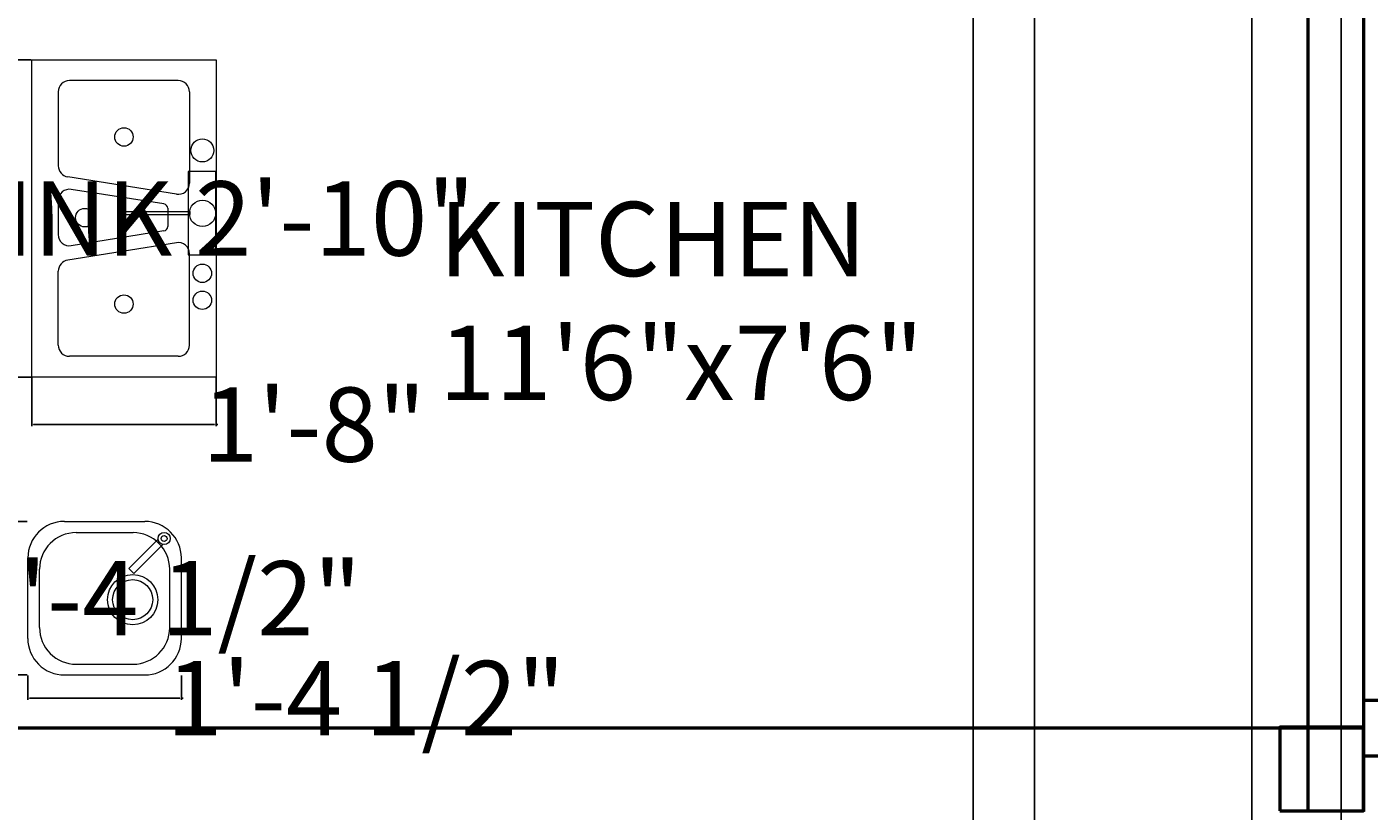
# Model space of a CAD drawing. Units: inches. Extents: x 1305 to 1889, y -508 to -5.
# Tile 3 of 8: x 1403 to 1548, y -389 to -305. Entities that reach past the tile are written whole.
import ezdxf

# ---------------------------------------------------------------- set-up
doc = ezdxf.new("R2010")
doc.units = ezdxf.units.IN
doc.header["$MEASUREMENT"] = 0
for name, color, linetype, lineweight in [('A-ANNO-DIMS', 2, 'Continuous', 18), ('A-AREA-IDEN', 7, 'Continuous', 25), ('A-COLS', 7, 'Continuous', 50), ('A-FLOR-FIXT', 9, 'Continuous', 18), ('A-WALL', 7, 'Continuous', 50)]:
    doc.layers.add(name, color=color, linetype=linetype, lineweight=lineweight)
doc.styles.get("Standard").update_dxf_attribs({"font": 'arial.ttf', "height": 8})
doc.dimstyles.get("Standard").update_dxf_attribs({"dimtxt": 0.18, "dimasz": 0.18, "dimexe": 0.18, "dimexo": 0.0625, "dimgap": 0.09, "dimtad": 0, "dimtih": 1, "dimtoh": 1, "dimzin": 0, "dimdsep": 46, "dimlunit": 4, "dimtxsty": 'Standard', "dimcen": 0.09, "dimadec": 0, "dimazin": 0, "dimtfac": 1, "dimtofl": 0, "dimtmove": 0, "dimatfit": 3, "dimfxl": 1, "dimtolj": 1, "dimtzin": 0, "dimarcsym": 0})

# ---------------------------------------------------------------- blocks, each defined once
blk = doc.blocks.new('A$C27EB6A15')
for p, q in [((0, 0), (0, 644.7)), ((0, 644.7), (1110.1, 644.7)), ((682.1, 643.4), (390.6, 643.4)), ((390.6, 643.4), (390.6, 547.6)), ((682.1, 547.6), (682.1, 643.4)), ((1110.1, 644.7), (1110.1, 0)), ((111.7, 551.5), (431.6, 551.5)), ((390.6, 547.6), (682.1, 547.6)), ((530.7, 328), (530.7, 553.3)), ((541.9, 552.9), (541.9, 328)), ((998.4, 551.5), (678.5, 551.5)), ((72.5, 512.3), (72.5, 132)), ((470.2, 506.2), (409.5, 125.9)), ((519.5, 475.4), (583.2, 475.4)), ((639.9, 506.2), (700.6, 125.9)), ((1037.5, 512.3), (1037.5, 132)), ((504.1, 462.2), (453.4, 137.6)), ((598.6, 462.2), (650.4, 137.8)), ((541.9, 328), (530.7, 328)), ((111.7, 92.9), (370.9, 92.9)), ((492.1, 92.5), (611.7, 92.5)), ((998.4, 92.9), (739.2, 92.9)), ((1110.1, 0), (0, 0))]:
    blk.add_line(p, q)
for centre, radius in [((317, 596.6), 40.3), ((537.2, 597.3), 45.9), ((747.1, 596.6), 32.3), ((841.3, 596.6), 32.3), ((269.9, 322.4), 32.3), ((854.7, 322.4), 32.3), ((552.2, 185.3), 32.3)]:
    blk.add_circle(centre, radius)
for centre, radius, start, end in [((111.7, 512.3), 39.1, 90, 180), ((431.6, 512.3), 39.1, 350.9343, 90), ((538.2, 591.7), 39.2, 259.3674, 275.2446), ((678.5, 512.3), 39.1, 90, 189.0657), ((998.4, 512.3), 39.1, 0, 90), ((519.5, 459.7), 15.7, 90, 171.1312), ((583.2, 459.7), 15.7, 9.0657, 90), ((111.7, 132), 39.1, 180, 270), ((370.9, 132), 39.1, 270, 350.9343), ((492.1, 131.6), 39.1, 171.1312, 270), ((611.7, 131.6), 39.1, 270, 9.0657), ((739.2, 132), 39.1, 189.0657, 270), ((998.4, 132), 39.1, 270, 0)]:
    blk.add_arc(centre, radius, start, end)
blk = doc.blocks.new('A$C027E3DAA')
for p, q in [((320, 419.7), (100, 419.7)), ((142.2, 289.7), (62.9, 369.3)), ((290.5, 387.8), (130.7, 387.8)), ((48.5, 356.2), (128.4, 276)), ((0, 100), (0, 319.7)), ((420, 100), (420, 319.7)), ((30.7, 132), (30.7, 287.8)), ((128.4, 276), (142.2, 289.7)), ((390.5, 132), (390.5, 287.8)), ((290.5, 32), (130.7, 32)), ((320, 0), (100, 0))]:
    blk.add_line(p, q)
for centre, radius in [((46.7, 372.6), 16.5), ((46.7, 372.6), 8.24), ((214, 286.7), 68.5), ((214, 286.7), 54.8)]:
    blk.add_circle(centre, radius)
for centre, start, end in [((100, 319.7), 90, 180), ((320, 319.7), 0, 90), ((130.7, 287.8), 90, 180), ((290.5, 287.8), 0, 90), ((130.7, 132), 180, 270), ((290.5, 132), 270, 0), ((100, 100), 180, 270), ((320, 100), 270, 0)]:
    blk.add_arc(centre, 100, start, end)
blk = doc.blocks.new('COL-9X9')
blk.add_lwpolyline([(0, 0), (9, 0), (9, 9), (0, 9)], close=True)
blk = doc.blocks.new('*D34')
at = {"layer": 'A-ANNO-DIMS', "color": 0, "lineweight": -2, "transparency": 16777216}
for p, q in [((1403.25, -358), (1400.66, -358)), ((1400.84, -358.18), (1400.84, -362.04)), ((1400.84, -374.35), (1400.84, -370.49)), ((1403.25, -374.53), (1400.66, -374.53))]:
    blk.add_line(p, q, dxfattribs=at)
at = {"layer": 'A-ANNO-DIMS', "color": 0, "transparency": 16777216}
for points in [[(1400.81, -358.18), (1400.87, -358.18), (1400.84, -358)], [(1400.81, -374.35), (1400.87, -374.35), (1400.84, -374.53)]]:
    blk.add_solid(points, dxfattribs=at)
at = {"layer": 'Defpoints', "color": 0, "transparency": 16777216}
for p in [(1403.32, -358), (1400.84, -374.53), (1403.32, -374.53)]:
    blk.add_point(p, dxfattribs=at)
at = {"layer": 'A-ANNO-DIMS', "color": 0, "transparency": 16777216, "insert": (1400.84, -366.27), "char_height": 8, "attachment_point": 5}
blk.add_mtext('\\A1;BASIN 1\'-4 1/2"', dxfattribs=at)
blk = doc.blocks.new('*D35')
at = {"layer": 'A-ANNO-DIMS', "color": 0, "lineweight": -2, "transparency": 16777216}
for p, q in [((1403.32, -374.6), (1403.32, -377.2)), ((1419.84, -374.6), (1419.84, -377.2)), ((1403.5, -377.02), (1419.66, -377.02)), ((1419.84, -377.02), (1420.02, -377.02))]:
    blk.add_line(p, q, dxfattribs=at)
at = {"layer": 'A-ANNO-DIMS', "color": 0, "transparency": 16777216}
for points in [[(1403.5, -376.99), (1403.5, -377.05), (1403.32, -377.02)], [(1419.66, -376.99), (1419.66, -377.05), (1419.84, -377.02)]]:
    blk.add_solid(points, dxfattribs=at)
at = {"layer": 'Defpoints', "color": 0, "transparency": 16777216}
for p in [(1403.32, -374.53), (1419.84, -374.53), (1419.84, -377.02)]:
    blk.add_point(p, dxfattribs=at)
at = {"layer": 'A-ANNO-DIMS', "color": 0, "transparency": 16777216, "insert": (1439.69, -377.02), "char_height": 8, "attachment_point": 5}
blk.add_mtext('\\A1;1\'-4 1/2"', dxfattribs=at)
blk = doc.blocks.new('*D44')
at = {"layer": 'A-ANNO-DIMS', "color": 0, "lineweight": -2, "transparency": 16777216}
for p, q in [((1403.68, -308.29), (1398.44, -308.29)), ((1398.62, -308.47), (1398.62, -321.14)), ((1398.62, -342.27), (1398.62, -329.59)), ((1403.68, -342.45), (1398.44, -342.45))]:
    blk.add_line(p, q, dxfattribs=at)
at = {"layer": 'A-ANNO-DIMS', "color": 0, "transparency": 16777216}
for points in [[(1398.59, -308.47), (1398.65, -308.47), (1398.62, -308.29)], [(1398.59, -342.27), (1398.65, -342.27), (1398.62, -342.45)]]:
    blk.add_solid(points, dxfattribs=at)
at = {"layer": 'Defpoints', "color": 0, "transparency": 16777216}
for p in [(1403.74, -308.29), (1398.62, -342.45), (1403.74, -342.45)]:
    blk.add_point(p, dxfattribs=at)
at = {"layer": 'A-ANNO-DIMS', "color": 0, "transparency": 16777216, "insert": (1398.62, -325.37), "char_height": 8, "attachment_point": 5}
blk.add_mtext('\\A1;KITCHEN SINK 2\'-10"', dxfattribs=at)
blk = doc.blocks.new('*D45')
at = {"layer": 'A-ANNO-DIMS', "color": 0, "lineweight": -2, "transparency": 16777216}
for p, q in [((1403.74, -342.51), (1403.74, -347.75)), ((1423.58, -342.51), (1423.58, -347.75)), ((1403.92, -347.57), (1423.4, -347.57)), ((1423.58, -347.57), (1423.76, -347.57))]:
    blk.add_line(p, q, dxfattribs=at)
at = {"layer": 'A-ANNO-DIMS', "color": 0, "transparency": 16777216}
for points in [[(1403.92, -347.54), (1403.92, -347.6), (1403.74, -347.57)], [(1423.4, -347.54), (1423.4, -347.6), (1423.58, -347.57)]]:
    blk.add_solid(points, dxfattribs=at)
at = {"layer": 'Defpoints', "color": 0, "transparency": 16777216}
for p in [(1403.74, -342.45), (1423.58, -342.45), (1423.58, -347.57)]:
    blk.add_point(p, dxfattribs=at)
at = {"layer": 'A-ANNO-DIMS', "color": 0, "transparency": 16777216, "insert": (1434.11, -347.57), "char_height": 8, "attachment_point": 5}
blk.add_mtext('\\A1;1\'-8"', dxfattribs=at)
blk = doc.blocks.new('*D55')
at = {"layer": 'A-ANNO-DIMS', "color": 0, "lineweight": -2, "transparency": 16777216}
for p, q in [((1511.68, -135.63), (1511.68, -493.26)), ((1544.68, -146.13), (1544.68, -493.26)), ((1511.86, -493.08), (1517.39, -493.08)), ((1544.5, -493.08), (1538.97, -493.08))]:
    blk.add_line(p, q, dxfattribs=at)
at = {"layer": 'A-ANNO-DIMS', "color": 0, "transparency": 16777216}
for points in [[(1511.86, -493.05), (1511.86, -493.11), (1511.68, -493.08)], [(1544.5, -493.05), (1544.5, -493.11), (1544.68, -493.08)]]:
    blk.add_solid(points, dxfattribs=at)
at = {"layer": 'Defpoints', "color": 0, "transparency": 16777216}
for p in [(1511.68, -135.57), (1544.68, -146.07), (1544.68, -493.08)]:
    blk.add_point(p, dxfattribs=at)
at = {"layer": 'A-ANNO-DIMS', "color": 0, "transparency": 16777216, "insert": (1528.18, -493.08), "char_height": 8, "attachment_point": 5}
blk.add_mtext('\\A1;2\'-9"', dxfattribs=at)
blk = doc.blocks.new('*D61')
at = {"layer": 'A-ANNO-DIMS', "color": 0, "lineweight": -2, "transparency": 16777216}
for p, q in [((1505.07, -290.3), (1505.07, -493.26)), ((1535.07, -290.3), (1535.07, -493.26)), ((1505.25, -493.08), (1509.28, -493.08)), ((1534.89, -493.08), (1530.87, -493.08))]:
    blk.add_line(p, q, dxfattribs=at)
at = {"layer": 'A-ANNO-DIMS', "color": 0, "transparency": 16777216}
for points in [[(1505.25, -493.05), (1505.25, -493.11), (1505.07, -493.08)], [(1534.89, -493.05), (1534.89, -493.11), (1535.07, -493.08)]]:
    blk.add_solid(points, dxfattribs=at)
at = {"layer": 'Defpoints', "color": 0, "transparency": 16777216}
for p in [(1505.07, -290.24), (1535.07, -290.24), (1535.07, -493.08)]:
    blk.add_point(p, dxfattribs=at)
at = {"layer": 'A-ANNO-DIMS', "color": 0, "transparency": 16777216, "insert": (1520.07, -493.08), "char_height": 8, "attachment_point": 5}
blk.add_mtext('\\A1;2\'-6"', dxfattribs=at)
blk = doc.blocks.new('*D69')
at = {"layer": 'A-ANNO-DIMS', "color": 0, "lineweight": -2, "transparency": 16777216}
for p, q in [((1547.07, -377.18), (1547.07, -85.83)), ((1547.25, -86.01), (1576.42, -86.01)), ((1576.6, -377.18), (1576.6, -85.83)), ((1576.6, -86.01), (1576.78, -86.01))]:
    blk.add_line(p, q, dxfattribs=at)
at = {"layer": 'A-ANNO-DIMS', "color": 0, "transparency": 16777216}
for points in [[(1547.25, -85.98), (1547.25, -86.04), (1547.07, -86.01)], [(1576.42, -85.98), (1576.42, -86.04), (1576.6, -86.01)]]:
    blk.add_solid(points, dxfattribs=at)
at = {"layer": 'Defpoints', "color": 0, "transparency": 16777216}
for p in [(1576.6, -86.01), (1547.07, -377.24), (1576.6, -377.24)]:
    blk.add_point(p, dxfattribs=at)
at = {"layer": 'A-ANNO-DIMS', "color": 0, "transparency": 16777216, "insert": (1596.89, -86.01), "char_height": 8, "attachment_point": 5}
blk.add_mtext('\\A1;2\'-5 1/2"', dxfattribs=at)

msp = doc.modelspace()

# ---------------------------------------------------------------- linework, layer by layer
at = {"layer": 'A-WALL'}
for p, q in [((1541.074, -248.321), (1541.074, -389.239)), ((1547.074, -248.321), (1547.074, -389.239)), ((1547.074, -377.239), (1637.074, -377.239)), ((1394.074, -380.239), (1547.074, -380.239)), ((1547.074, -383.239), (1637.074, -383.239))]:
    msp.add_line(p, q, dxfattribs=at)

# ---------------------------------------------------------------- block references
at = {"layer": 'A-COLS'}
msp.add_blockref('COL-9X9', (1538.072, -389.164), dxfattribs=at)
at = {"layer": 'A-FLOR-FIXT', "rotation": 270}
for name, p, xscale, yscale, zscale in [('A$C27EB6A15', (1403.742, -308.29), 0.0307684835218557, 0.0307684835218557, 0.0307684835218557), ('A$C027E3DAA', (1403.316, -357.999), 0.0393700787401575, 0.0393700787401575, 0.0393700787401575)]:
    msp.add_blockref(name, p, dxfattribs=dict(at, xscale=xscale, yscale=yscale, zscale=zscale))

# ---------------------------------------------------------------- texts
at = {"layer": 'A-AREA-IDEN', "insert": (1447.573, -323.586), "char_height": 8, "attachment_point": 1}
msp.add_mtext_dynamic_manual_height_columns('KITCHEN \\P11\'6"x7\'6"', width=69.27903, gutter_width=40, heights=[0], dxfattribs=at)

# ---------------------------------------------------------------- dimensions: what is measured, and where the dimension line sits
at = {"layer": 'A-ANNO-DIMS'}
for base, p1, p2, picture, middle in [((1576.598, -86.014), (1547.074, -377.239), (1576.598, -377.239), '*D69', (1596.889, -86.014)), ((1544.679, -493.076), (1511.679, -135.569), (1544.679, -146.069), '*D55', (1528.179, -493.076)), ((1535.074, -493.076), (1505.074, -290.239), (1535.074, -290.239), '*D61', (1520.074, -493.076)), ((1423.579, -347.569), (1403.742, -342.445), (1423.579, -342.445), '*D45', (1434.105, -347.569)), ((1419.842, -377.015), (1403.316, -374.535), (1419.842, -374.535), '*D35', (1439.689, -377.015))]:
    dim = msp.add_linear_dim(base=base, p1=p1, p2=p2, dimstyle='Standard', override={"dimdec": 1, "dimlfac": 1, "dimrnd": 0, "dimzin": 1, "dimdsep": 46, "dimlunit": 4, "dimfrac": 2}, dxfattribs=at)
    dim.commit()
    dim.dimension.update_dxf_attribs({"geometry": picture, "text_midpoint": middle})
for base, p1, p2, text, picture, middle in [((1398.618, -342.445), (1403.742, -308.29), (1403.742, -342.445), 'KITCHEN SINK <>', '*D44', (1398.618, -325.368)), ((1400.836, -374.535), (1403.316, -357.999), (1403.316, -374.535), 'BASIN <>', '*D34', (1400.836, -366.267))]:
    dim = msp.add_linear_dim(base=base, p1=p1, p2=p2, angle=270, text=text, dimstyle='Standard', override={"dimdec": 1, "dimlfac": 1, "dimrnd": 0, "dimzin": 1, "dimdsep": 46, "dimlunit": 4, "dimfrac": 2}, dxfattribs=at)
    dim.commit()
    dim.dimension.update_dxf_attribs({"geometry": picture, "text_midpoint": middle})

doc.saveas('drawing.dxf')
